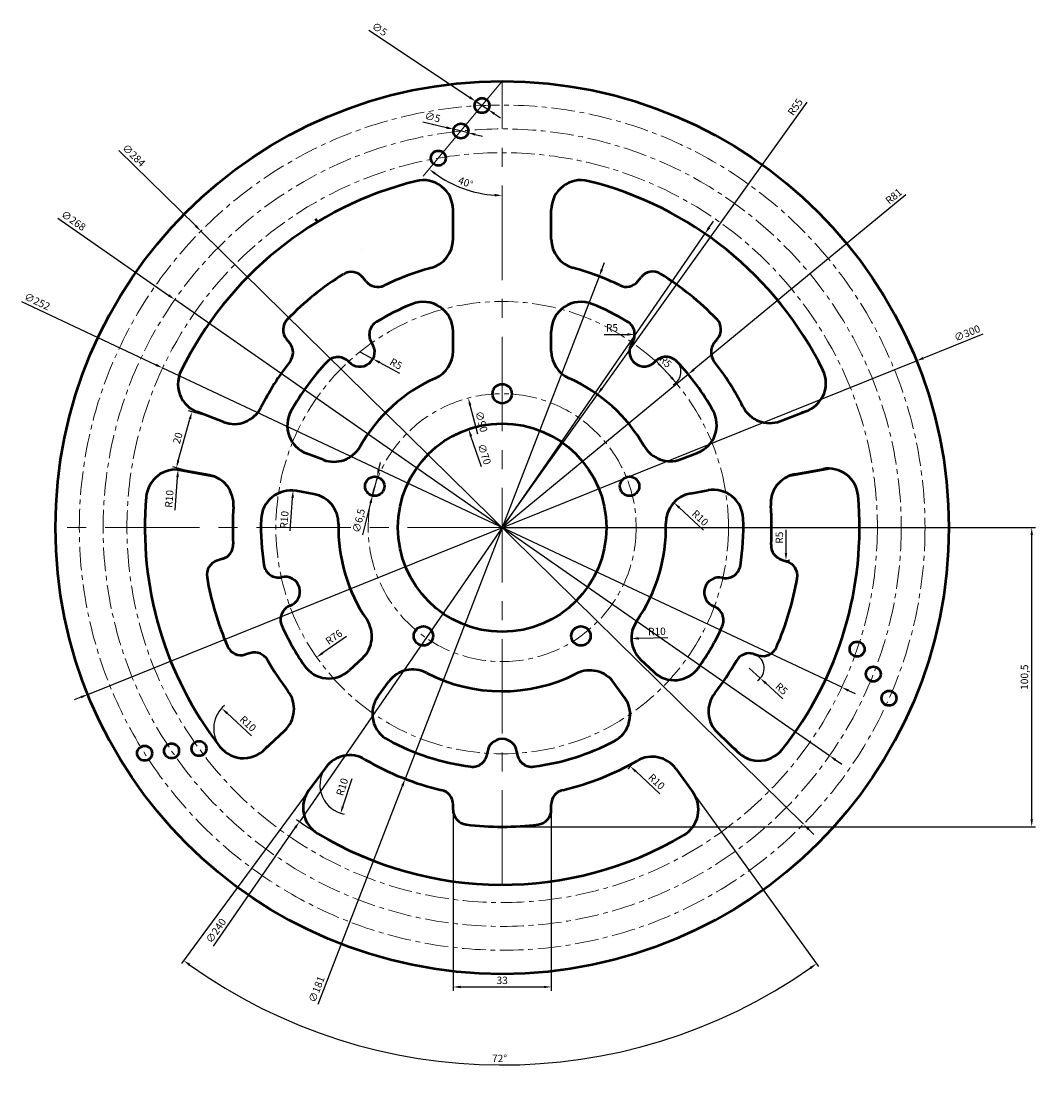
# Model space of a CAD drawing. Units: millimetres. Extents: x 2992 to 3333, y 1221 to 1583.
import ezdxf

# ---------------------------------------------------------------- set-up
doc = ezdxf.new("R2010")
doc.units = ezdxf.units.MM
doc.linetypes.add('CENTER', pattern=[50.8, 31.75, -6.35, 6.35, -6.35])
for name, color, linetype, lineweight in [('M-CNTR', 4, 'CENTER', 18), ('M-CONS', 8, 'Continuous', 13), ('M-DIMS', 2, 'Continuous', 25), ('M-OUTL', 7, 'Continuous', 50)]:
    doc.layers.add(name, color=color, linetype=linetype, lineweight=lineweight)
doc.styles.get("Standard").update_dxf_attribs({"font": 'arial.ttf'})
doc.dimstyles.new('ISO-25', dxfattribs={"dimtxt": 2.5, "dimasz": 2.5, "dimexe": 1.25, "dimexo": 0.625, "dimtad": 1, "dimtxsty": 'Standard', "dimcen": 2.5, "dimadec": 0, "dimazin": 0, "dimtfac": 1, "dimtmove": 0, "dimatfit": 3, "dimfxl": 1, "dimarcsym": 0})

# ---------------------------------------------------------------- blocks, each defined once
blk = doc.blocks.new('*D1')
at = {"layer": 'Defpoints', "color": 0, "transparency": 16777216}
for p in [(3137.05, 1317.59), (3170.04, 1317.59), (3170.04, 1258.36)]:
    blk.add_point(p, dxfattribs=at)
at = {"layer": 'M-DIMS', "color": 0, "lineweight": -2, "transparency": 16777216}
for p, q in [((3137.05, 1316.96), (3137.05, 1257.11)), ((3170.04, 1316.96), (3170.04, 1257.11)), ((3139.55, 1258.36), (3167.54, 1258.36))]:
    blk.add_line(p, q, dxfattribs=at)
at = {"layer": 'M-DIMS', "color": 0, "transparency": 16777216}
for points in [[(3139.55, 1258.77), (3139.55, 1257.94), (3137.05, 1258.36)], [(3167.54, 1258.77), (3167.54, 1257.94), (3170.04, 1258.36)]]:
    blk.add_solid(points, dxfattribs=at)
at = {"layer": 'M-DIMS', "color": 0, "transparency": 16777216, "insert": (3153.54, 1260.26), "char_height": 2.5, "attachment_point": 5}
blk.add_mtext('33', dxfattribs=at)
blk = doc.blocks.new('*D2')
at = {"layer": 'Defpoints', "color": 0, "transparency": 16777216}
for p in [(3049.35, 1451.62), (3055.58, 1449.88), (3050.33, 1431.07)]:
    blk.add_point(p, dxfattribs=at)
at = {"layer": 'M-DIMS', "color": 0, "lineweight": -2, "transparency": 16777216}
for p, q in [((3054.98, 1450.05), (3048.15, 1451.95)), ((3044.78, 1435.21), (3048.68, 1449.21)), ((3049.73, 1431.24), (3042.9, 1433.14))]:
    blk.add_line(p, q, dxfattribs=at)
at = {"layer": 'M-DIMS', "color": 0, "transparency": 16777216}
for points in [[(3048.28, 1449.32), (3049.08, 1449.1), (3049.35, 1451.62)], [(3044.38, 1435.33), (3045.18, 1435.1), (3044.1, 1432.81)]]:
    blk.add_solid(points, dxfattribs=at)
at = {"layer": 'M-DIMS', "color": 0, "transparency": 16777216, "insert": (3044.9, 1442.72), "char_height": 2.5, "attachment_point": 5, "rotation": 74.4122}
blk.add_mtext('20', dxfattribs=at)
blk = doc.blocks.new('*D3')
at = {"layer": 'Defpoints', "color": 0, "transparency": 16777216}
for p in [(3153.54, 1412.71), (3331.37, 1412.71), (3153.54, 1312.21)]:
    blk.add_point(p, dxfattribs=at)
at = {"layer": 'M-DIMS', "color": 0, "lineweight": -2, "transparency": 16777216}
for p, q in [((3154.16, 1412.71), (3332.62, 1412.71)), ((3331.37, 1314.71), (3331.37, 1410.21)), ((3154.16, 1312.21), (3332.62, 1312.21))]:
    blk.add_line(p, q, dxfattribs=at)
at = {"layer": 'M-DIMS', "color": 0, "transparency": 16777216}
for points in [[(3330.96, 1410.21), (3331.79, 1410.21), (3331.37, 1412.71)], [(3330.96, 1314.71), (3331.79, 1314.71), (3331.37, 1312.21)]]:
    blk.add_solid(points, dxfattribs=at)
at = {"layer": 'M-DIMS', "color": 0, "transparency": 16777216, "insert": (3329.25, 1362.46), "char_height": 2.5, "attachment_point": 5, "rotation": 90}
blk.add_mtext('100,5', dxfattribs=at)
blk = doc.blocks.new('*D4')
at = {"layer": 'Defpoints', "color": 0, "transparency": 16777216}
for p in [(3292.68, 1468.75), (3014.4, 1356.66)]:
    blk.add_point(p, dxfattribs=at)
at = {"layer": 'M-DIMS', "color": 0, "lineweight": -2, "transparency": 16777216}
for p, q in [((3314.94, 1477.72), (3294.99, 1469.69)), ((3014.4, 1356.66), (3292.68, 1468.75)), ((3012.08, 1355.73), (3009.76, 1354.8))]:
    blk.add_line(p, q, dxfattribs=at)
at = {"layer": 'M-DIMS', "color": 0, "transparency": 16777216}
for points in [[(3294.84, 1470.07), (3295.15, 1469.3), (3292.68, 1468.75)], [(3011.93, 1356.12), (3012.24, 1355.34), (3014.4, 1356.66)]]:
    blk.add_solid(points, dxfattribs=at)
at = {"layer": 'M-DIMS', "color": 0, "transparency": 16777216, "insert": (3309.8, 1477.78), "char_height": 2.5, "attachment_point": 5, "rotation": 21.9393}
blk.add_mtext('∅300', dxfattribs=at)
blk = doc.blocks.new('*D5')
at = {"layer": 'Defpoints', "color": 0, "transparency": 16777216}
for p in [(3144.69, 1555.93), (3148.85, 1553.16)]:
    blk.add_point(p, dxfattribs=at)
at = {"layer": 'M-DIMS', "color": 0, "lineweight": -2, "transparency": 16777216}
for p, q in [((3108.77, 1579.86), (3142.6, 1557.32)), ((3148.85, 1553.16), (3144.69, 1555.93)), ((3150.93, 1551.77), (3153.01, 1550.39))]:
    blk.add_line(p, q, dxfattribs=at)
at = {"layer": 'M-DIMS', "color": 0, "transparency": 16777216}
for points in [[(3142.84, 1557.67), (3142.37, 1556.97), (3144.69, 1555.93)], [(3151.16, 1552.12), (3150.7, 1551.43), (3148.85, 1553.16)]]:
    blk.add_solid(points, dxfattribs=at)
at = {"layer": 'M-DIMS', "color": 0, "transparency": 16777216, "insert": (3112.2, 1579.94), "char_height": 2.5, "attachment_point": 5, "rotation": 326.3304}
blk.add_mtext('∅5', dxfattribs=at)
blk = doc.blocks.new('*D6')
at = {"layer": 'Defpoints', "color": 0, "transparency": 16777216}
for p in [(3052.39, 1512.37), (3254.69, 1313.05)]:
    blk.add_point(p, dxfattribs=at)
at = {"layer": 'M-DIMS', "color": 0, "lineweight": -2, "transparency": 16777216}
for p, q in [((3024.86, 1539.49), (3050.61, 1514.13)), ((3254.69, 1313.05), (3052.39, 1512.37)), ((3256.47, 1311.29), (3258.25, 1309.54))]:
    blk.add_line(p, q, dxfattribs=at)
at = {"layer": 'M-DIMS', "color": 0, "transparency": 16777216}
for points in [[(3050.9, 1514.42), (3050.31, 1513.83), (3052.39, 1512.37)], [(3256.76, 1311.59), (3256.18, 1310.99), (3254.69, 1313.05)]]:
    blk.add_solid(points, dxfattribs=at)
at = {"layer": 'M-DIMS', "color": 0, "transparency": 16777216, "insert": (3029.62, 1537.57), "char_height": 2.5, "attachment_point": 5, "rotation": 315.4245}
blk.add_mtext('∅284', dxfattribs=at)
blk = doc.blocks.new('*D7')
at = {"layer": 'Defpoints', "color": 0, "transparency": 16777216}
for p in [(3043.61, 1489.34), (3263.46, 1336.07)]:
    blk.add_point(p, dxfattribs=at)
at = {"layer": 'M-DIMS', "color": 0, "lineweight": -2, "transparency": 16777216}
for p, q in [((3004.36, 1516.71), (3041.56, 1490.77)), ((3263.46, 1336.07), (3043.61, 1489.34)), ((3265.51, 1334.64), (3267.56, 1333.21))]:
    blk.add_line(p, q, dxfattribs=at)
at = {"layer": 'M-DIMS', "color": 0, "transparency": 16777216}
for points in [[(3041.8, 1491.11), (3041.33, 1490.43), (3043.61, 1489.34)], [(3265.75, 1334.99), (3265.27, 1334.3), (3263.46, 1336.07)]]:
    blk.add_solid(points, dxfattribs=at)
at = {"layer": 'M-DIMS', "color": 0, "transparency": 16777216, "insert": (3009.39, 1515.61), "char_height": 2.5, "attachment_point": 5, "rotation": 325.1175}
blk.add_mtext('∅268', dxfattribs=at)
blk = doc.blocks.new('*D8')
at = {"layer": 'Defpoints', "color": 0, "transparency": 16777216}
for p in [(3039.53, 1466.35), (3267.55, 1359.06)]:
    blk.add_point(p, dxfattribs=at)
at = {"layer": 'M-DIMS', "color": 0, "lineweight": -2, "transparency": 16777216}
for p, q in [((2992.14, 1488.66), (3037.27, 1467.42)), ((3267.55, 1359.06), (3039.53, 1466.35)), ((3269.81, 1358), (3272.07, 1356.93))]:
    blk.add_line(p, q, dxfattribs=at)
at = {"layer": 'M-DIMS', "color": 0, "transparency": 16777216}
for points in [[(3037.44, 1467.8), (3037.09, 1467.04), (3039.53, 1466.35)], [(3269.99, 1358.37), (3269.63, 1357.62), (3267.55, 1359.06)]]:
    blk.add_solid(points, dxfattribs=at)
at = {"layer": 'M-DIMS', "color": 0, "transparency": 16777216, "insert": (2997.26, 1488.42), "char_height": 2.5, "attachment_point": 5, "rotation": 334.8007}
blk.add_mtext('∅252', dxfattribs=at)
blk = doc.blocks.new('*D9')
at = {"layer": 'Defpoints', "color": 0, "transparency": 16777216}
for p in [(3221.63, 1511.52), (3085.45, 1313.9)]:
    blk.add_point(p, dxfattribs=at)
at = {"layer": 'M-DIMS', "color": 0, "lineweight": -2, "transparency": 16777216}
for p, q in [((3223.05, 1513.58), (3224.46, 1515.64)), ((3221.63, 1511.52), (3085.45, 1313.9)), ((3056.62, 1272.06), (3084.03, 1311.84))]:
    blk.add_line(p, q, dxfattribs=at)
blk.add_arc((3153.54, 1412.71), 120, 234.8334, 238.5826, dxfattribs=at)
at = {"layer": 'M-DIMS', "color": 0, "transparency": 16777216}
for points in [[(3222.7, 1513.82), (3223.39, 1513.34), (3221.63, 1511.52)], [(3083.69, 1312.07), (3084.37, 1311.6), (3085.45, 1313.9)]]:
    blk.add_solid(points, dxfattribs=at)
at = {"layer": 'M-DIMS', "color": 0, "transparency": 16777216, "insert": (3057.69, 1277.09), "char_height": 2.5, "attachment_point": 5, "rotation": 55.4302}
blk.add_mtext('∅240', dxfattribs=at)
blk = doc.blocks.new('*D10')
at = {"layer": 'Defpoints', "color": 0, "transparency": 16777216}
for p in [(3186.12, 1497.14), (3120.95, 1328.28)]:
    blk.add_point(p, dxfattribs=at)
at = {"layer": 'M-DIMS', "color": 0, "lineweight": -2, "transparency": 16777216}
for p, q in [((3187.02, 1499.47), (3187.92, 1501.8)), ((3186.12, 1497.14), (3120.95, 1328.28)), ((3091.73, 1252.54), (3120.05, 1325.95))]:
    blk.add_line(p, q, dxfattribs=at)
at = {"layer": 'M-DIMS', "color": 0, "transparency": 16777216}
for points in [[(3186.63, 1499.62), (3187.41, 1499.32), (3186.12, 1497.14)], [(3119.67, 1326.1), (3120.44, 1325.79), (3120.95, 1328.28)]]:
    blk.add_solid(points, dxfattribs=at)
at = {"layer": 'M-DIMS', "color": 0, "transparency": 16777216, "insert": (3091.51, 1257.46), "char_height": 2.5, "attachment_point": 5, "rotation": 68.8971}
blk.add_mtext('∅181', dxfattribs=at)
blk = doc.blocks.new('*D11')
at = {"layer": 'Defpoints', "color": 0, "transparency": 16777216}
for p in [(3105.74, 1471.79), (3110.14, 1469.42)]:
    blk.add_point(p, dxfattribs=at)
at = {"layer": 'M-DIMS', "color": 0, "lineweight": -2, "transparency": 16777216}
for p, q in [((3105.74, 1471.79), (3110.14, 1469.42)), ((3119.2, 1464.53), (3112.34, 1468.23))]:
    blk.add_line(p, q, dxfattribs=at)
at = {"layer": 'M-DIMS', "color": 0, "transparency": 16777216}
blk.add_solid([(3112.54, 1468.6), (3112.14, 1467.87), (3110.14, 1469.42)], dxfattribs=at)
at = {"layer": 'M-DIMS', "color": 0, "transparency": 16777216, "insert": (3117.77, 1467.46), "char_height": 2.5, "attachment_point": 5, "rotation": 331.6611}
blk.add_mtext('R5', dxfattribs=at)
blk = doc.blocks.new('*D12')
at = {"layer": 'Defpoints', "color": 0, "transparency": 16777216}
for p in [(3193.06, 1477.62), (3198.06, 1477.62)]:
    blk.add_point(p, dxfattribs=at)
at = {"layer": 'M-DIMS', "color": 0, "lineweight": -2, "transparency": 16777216}
blk.add_line((3187.76, 1477.62), (3195.56, 1477.62), dxfattribs=at)
at = {"layer": 'M-DIMS', "color": 0, "transparency": 16777216}
blk.add_solid([(3195.56, 1478.04), (3195.56, 1477.21), (3198.06, 1477.62)], dxfattribs=at)
at = {"layer": 'M-DIMS', "color": 0, "transparency": 16777216, "insert": (3190.41, 1479.52), "char_height": 2.5, "attachment_point": 5}
blk.add_mtext('R5', dxfattribs=at)
blk = doc.blocks.new('*D13')
at = {"layer": 'Defpoints', "color": 0, "transparency": 16777216}
for p in [(3208.59, 1465.1), (3211.98, 1461.42)]:
    blk.add_point(p, dxfattribs=at)
at = {"layer": 'M-DIMS', "color": 0, "lineweight": -2, "transparency": 16777216}
blk.add_line((3205.01, 1469), (3210.29, 1463.26), dxfattribs=at)
blk.add_arc((3208.59, 1465.1), 5, 298.2777, 36.4174, dxfattribs=at)
at = {"layer": 'M-DIMS', "color": 0, "transparency": 16777216}
blk.add_solid([(3210.59, 1463.54), (3209.98, 1462.98), (3211.98, 1461.42)], dxfattribs=at)
at = {"layer": 'M-DIMS', "color": 0, "transparency": 16777216, "insert": (3208.2, 1468.33), "char_height": 2.5, "attachment_point": 5, "rotation": 312.6017}
blk.add_mtext('R5', dxfattribs=at)
blk = doc.blocks.new('*D14')
at = {"layer": 'Defpoints', "color": 0, "transparency": 16777216}
for p in [(3211.19, 1421.13), (3218.52, 1414.33)]:
    blk.add_point(p, dxfattribs=at)
at = {"layer": 'M-DIMS', "color": 0, "lineweight": -2, "transparency": 16777216}
blk.add_line((3221.16, 1411.87), (3213.02, 1419.43), dxfattribs=at)
at = {"layer": 'M-DIMS', "color": 0, "transparency": 16777216}
blk.add_solid([(3213.3, 1419.73), (3212.74, 1419.12), (3211.19, 1421.13)], dxfattribs=at)
at = {"layer": 'M-DIMS', "color": 0, "transparency": 16777216, "insert": (3219.81, 1415.72), "char_height": 2.5, "attachment_point": 5, "rotation": 317.1429}
blk.add_mtext('R10', dxfattribs=at)
blk = doc.blocks.new('*D15')
at = {"layer": 'Defpoints', "color": 0, "transparency": 16777216}
for p in [(3196.93, 1375.45), (3206.93, 1375.64)]:
    blk.add_point(p, dxfattribs=at)
at = {"layer": 'M-DIMS', "color": 0, "lineweight": -2, "transparency": 16777216}
blk.add_line((3209.15, 1375.68), (3199.43, 1375.5), dxfattribs=at)
at = {"layer": 'M-DIMS', "color": 0, "transparency": 16777216}
blk.add_solid([(3199.42, 1375.92), (3199.44, 1375.08), (3196.93, 1375.45)], dxfattribs=at)
at = {"layer": 'M-DIMS', "color": 0, "transparency": 16777216, "insert": (3205.5, 1377.51), "char_height": 2.5, "attachment_point": 5, "rotation": 1.0474}
blk.add_mtext('R10', dxfattribs=at)
blk = doc.blocks.new('*D16')
at = {"layer": 'Defpoints', "color": 0, "transparency": 16777216}
for p in [(3153.54, 1412.71), (3091.25, 1369.16)]:
    blk.add_point(p, dxfattribs=at)
at = {"layer": 'M-DIMS', "color": 0, "lineweight": -2, "transparency": 16777216}
blk.add_line((3101.27, 1376.17), (3093.3, 1370.59), dxfattribs=at)
at = {"layer": 'M-DIMS', "color": 0, "transparency": 16777216}
blk.add_solid([(3093.06, 1370.94), (3093.54, 1370.25), (3091.25, 1369.16)], dxfattribs=at)
at = {"layer": 'M-DIMS', "color": 0, "transparency": 16777216, "insert": (3097.22, 1375.65), "char_height": 2.5, "attachment_point": 5, "rotation": 34.9576}
blk.add_mtext('R76', dxfattribs=at)
blk = doc.blocks.new('*D17')
at = {"layer": 'Defpoints', "color": 0, "transparency": 16777216}
for p in [(3083.33, 1425.15), (3082.58, 1415.17)]:
    blk.add_point(p, dxfattribs=at)
at = {"layer": 'M-DIMS', "color": 0, "lineweight": -2, "transparency": 16777216}
blk.add_line((3082.31, 1411.58), (3083.14, 1422.65), dxfattribs=at)
at = {"layer": 'M-DIMS', "color": 0, "transparency": 16777216}
blk.add_solid([(3082.73, 1422.69), (3083.56, 1422.62), (3083.33, 1425.15)], dxfattribs=at)
at = {"layer": 'M-DIMS', "color": 0, "transparency": 16777216, "insert": (3080.69, 1415.32), "char_height": 2.5, "attachment_point": 5, "rotation": 85.7143}
blk.add_mtext('R10', dxfattribs=at)
blk = doc.blocks.new('*D18')
at = {"layer": 'Defpoints', "color": 0, "transparency": 16777216}
for p in [(3044.7, 1432.18), (3043.95, 1422.2)]:
    blk.add_point(p, dxfattribs=at)
at = {"layer": 'M-DIMS', "color": 0, "lineweight": -2, "transparency": 16777216}
blk.add_line((3043.68, 1418.61), (3044.51, 1429.68), dxfattribs=at)
at = {"layer": 'M-DIMS', "color": 0, "transparency": 16777216}
blk.add_solid([(3044.09, 1429.72), (3044.93, 1429.65), (3044.7, 1432.18)], dxfattribs=at)
at = {"layer": 'M-DIMS', "color": 0, "transparency": 16777216, "insert": (3042.05, 1422.35), "char_height": 2.5, "attachment_point": 5, "rotation": 85.7143}
blk.add_mtext('R10', dxfattribs=at)
blk = doc.blocks.new('*D19')
at = {"layer": 'Defpoints', "color": 0, "transparency": 16777216}
for p in [(3059.34, 1352.03), (3066.67, 1345.23)]:
    blk.add_point(p, dxfattribs=at)
at = {"layer": 'M-DIMS', "color": 0, "lineweight": -2, "transparency": 16777216}
blk.add_line((3069.31, 1342.78), (3061.17, 1350.33), dxfattribs=at)
blk.add_arc((3066.67, 1345.23), 10, 129.9809, 214.2575, dxfattribs=at)
at = {"layer": 'M-DIMS', "color": 0, "transparency": 16777216}
blk.add_solid([(3061.45, 1350.64), (3060.89, 1350.03), (3059.34, 1352.03)], dxfattribs=at)
at = {"layer": 'M-DIMS', "color": 0, "transparency": 16777216, "insert": (3067.96, 1346.62), "char_height": 2.5, "attachment_point": 5, "rotation": 317.1429}
blk.add_mtext('R10', dxfattribs=at)
blk = doc.blocks.new('*D20')
at = {"layer": 'Defpoints', "color": 0, "transparency": 16777216}
for p in [(3102.34, 1326.23), (3099.28, 1316.71)]:
    blk.add_point(p, dxfattribs=at)
at = {"layer": 'M-DIMS', "color": 0, "lineweight": -2, "transparency": 16777216}
blk.add_line((3103.02, 1328.33), (3100.04, 1319.09), dxfattribs=at)
blk.add_arc((3102.34, 1326.23), 10, 147.246, 259.3056, dxfattribs=at)
at = {"layer": 'M-DIMS', "color": 0, "transparency": 16777216}
blk.add_solid([(3099.65, 1319.21), (3100.44, 1318.96), (3099.28, 1316.71)], dxfattribs=at)
at = {"layer": 'M-DIMS', "color": 0, "transparency": 16777216, "insert": (3100.11, 1325.48), "char_height": 2.5, "attachment_point": 5, "rotation": 72.1436}
blk.add_mtext('R10', dxfattribs=at)
blk = doc.blocks.new('*D21')
at = {"layer": 'Defpoints', "color": 0, "transparency": 16777216}
for p in [(3196.54, 1332.52), (3203.87, 1325.72)]:
    blk.add_point(p, dxfattribs=at)
at = {"layer": 'M-DIMS', "color": 0, "lineweight": -2, "transparency": 16777216}
blk.add_line((3206.52, 1323.27), (3198.37, 1330.82), dxfattribs=at)
blk.add_arc((3203.87, 1325.72), 10, 123.6362, 144.3048, dxfattribs=at)
at = {"layer": 'M-DIMS', "color": 0, "transparency": 16777216}
blk.add_solid([(3198.66, 1331.13), (3198.09, 1330.52), (3196.54, 1332.52)], dxfattribs=at)
at = {"layer": 'M-DIMS', "color": 0, "transparency": 16777216, "insert": (3205.17, 1327.11), "char_height": 2.5, "attachment_point": 5, "rotation": 317.1429}
blk.add_mtext('R10', dxfattribs=at)
blk = doc.blocks.new('*D22')
at = {"layer": 'Defpoints', "color": 0, "transparency": 16777216}
for p in [(3248.85, 1406.68), (3248.85, 1401.68)]:
    blk.add_point(p, dxfattribs=at)
at = {"layer": 'M-DIMS', "color": 0, "lineweight": -2, "transparency": 16777216}
blk.add_line((3248.85, 1411.98), (3248.85, 1404.18), dxfattribs=at)
blk.add_arc((3248.85, 1406.68), 5, 260.5307, 284.3239, dxfattribs=at)
at = {"layer": 'M-DIMS', "color": 0, "transparency": 16777216}
blk.add_solid([(3248.43, 1404.18), (3249.26, 1404.18), (3248.85, 1401.68)], dxfattribs=at)
at = {"layer": 'M-DIMS', "color": 0, "transparency": 16777216, "insert": (3246.95, 1409.33), "char_height": 2.5, "attachment_point": 5, "rotation": 90}
blk.add_mtext('R5', dxfattribs=at)
blk = doc.blocks.new('*D23')
at = {"layer": 'Defpoints', "color": 0, "transparency": 16777216}
for p in [(3236.54, 1365.48), (3240.23, 1362.1)]:
    blk.add_point(p, dxfattribs=at)
at = {"layer": 'M-DIMS', "color": 0, "lineweight": -2, "transparency": 16777216}
for p, q in [((3236.54, 1365.48), (3240.23, 1362.1)), ((3247.83, 1355.15), (3242.08, 1360.42))]:
    blk.add_line(p, q, dxfattribs=at)
blk.add_arc((3236.54, 1365.48), 5, 303.2437, 66.2068, dxfattribs=at)
at = {"layer": 'M-DIMS', "color": 0, "transparency": 16777216}
blk.add_solid([(3242.36, 1360.72), (3241.8, 1360.11), (3240.23, 1362.1)], dxfattribs=at)
at = {"layer": 'M-DIMS', "color": 0, "transparency": 16777216, "insert": (3247.16, 1358.34), "char_height": 2.5, "attachment_point": 5, "rotation": 317.5677}
blk.add_mtext('R5', dxfattribs=at)
blk = doc.blocks.new('*D24')
at = {"layer": 'Defpoints', "color": 0, "transparency": 16777216}
for p in [(3216.02, 1464.25), (3153.54, 1412.71)]:
    blk.add_point(p, dxfattribs=at)
at = {"layer": 'M-DIMS', "color": 0, "lineweight": -2, "transparency": 16777216}
for p, q in [((3289.05, 1524.5), (3217.95, 1465.84)), ((3153.54, 1412.71), (3216.02, 1464.25))]:
    blk.add_line(p, q, dxfattribs=at)
at = {"layer": 'M-DIMS', "color": 0, "transparency": 16777216}
blk.add_solid([(3217.68, 1466.17), (3218.21, 1465.52), (3216.02, 1464.25)], dxfattribs=at)
at = {"layer": 'M-DIMS', "color": 0, "transparency": 16777216, "insert": (3285.24, 1523.82), "char_height": 2.5, "attachment_point": 5, "rotation": 39.5211}
blk.add_mtext('R81', dxfattribs=at)
blk = doc.blocks.new('*D25')
at = {"layer": 'Defpoints', "color": 0, "transparency": 16777216}
for p in [(3185.55, 1457.44), (3153.54, 1412.71)]:
    blk.add_point(p, dxfattribs=at)
at = {"layer": 'M-DIMS', "color": 0, "lineweight": -2, "transparency": 16777216}
for p, q in [((3255.88, 1555.72), (3187, 1459.47)), ((3153.54, 1412.71), (3185.55, 1457.44))]:
    blk.add_line(p, q, dxfattribs=at)
at = {"layer": 'M-DIMS', "color": 0, "transparency": 16777216}
blk.add_solid([(3186.66, 1459.71), (3187.34, 1459.23), (3185.55, 1457.44)], dxfattribs=at)
at = {"layer": 'M-DIMS', "color": 0, "transparency": 16777216, "insert": (3252.23, 1553.88), "char_height": 2.5, "attachment_point": 5, "rotation": 54.4123}
blk.add_mtext('R55', dxfattribs=at)
blk = doc.blocks.new('*D26')
at = {"layer": 'Defpoints', "color": 0, "transparency": 16777216}
for p in [(3142.26, 1445.84), (3164.81, 1379.57)]:
    blk.add_point(p, dxfattribs=at)
at = {"layer": 'M-DIMS', "color": 0, "lineweight": -2, "transparency": 16777216}
blk.add_line((3146.6, 1433.09), (3143.07, 1443.47), dxfattribs=at)
at = {"layer": 'M-DIMS', "color": 0, "transparency": 16777216}
blk.add_solid([(3143.46, 1443.61), (3142.67, 1443.34), (3142.26, 1445.84)], dxfattribs=at)
at = {"layer": 'M-DIMS', "color": 0, "transparency": 16777216, "insert": (3147.25, 1437.3), "char_height": 2.5, "attachment_point": 5, "rotation": 288.7953}
blk.add_mtext('∅70', dxfattribs=at)
blk = doc.blocks.new('*D27')
at = {"layer": 'Defpoints', "color": 0, "transparency": 16777216}
for p in [(3142.15, 1456.24), (3164.92, 1369.17)]:
    blk.add_point(p, dxfattribs=at)
at = {"layer": 'M-DIMS', "color": 0, "lineweight": -2, "transparency": 16777216}
blk.add_line((3145.33, 1444.11), (3142.79, 1453.83), dxfattribs=at)
at = {"layer": 'M-DIMS', "color": 0, "transparency": 16777216}
blk.add_solid([(3143.19, 1453.93), (3142.38, 1453.72), (3142.15, 1456.24)], dxfattribs=at)
at = {"layer": 'M-DIMS', "color": 0, "transparency": 16777216, "insert": (3146.28, 1448.26), "char_height": 2.5, "attachment_point": 5, "rotation": 284.6536}
blk.add_mtext('∅90', dxfattribs=at)
blk = doc.blocks.new('*D28')
at = {"layer": 'Defpoints', "color": 0, "transparency": 16777216}
for p in [(3094.29, 1332.15), (3211.99, 1331.57), (3088.63, 1324.46), (3217.56, 1323.82), (3115.07, 1236.28)]:
    blk.add_point(p, dxfattribs=at)
at = {"layer": 'M-DIMS', "color": 0, "lineweight": -2, "transparency": 16777216}
for p, q in [((3088.26, 1323.96), (3045.81, 1266.24)), ((3217.93, 1323.31), (3259.81, 1265.18))]:
    blk.add_line(p, q, dxfattribs=at)
blk.add_arc((3153.54, 1412.71), 180.57, 234.4583, 304.9725, dxfattribs=at)
at = {"layer": 'M-DIMS', "color": 0, "transparency": 16777216}
for points in [[(3048.33, 1265.44), (3048.82, 1266.12), (3046.55, 1267.25)], [(3256.8, 1265.08), (3257.28, 1264.4), (3259.08, 1266.19)]]:
    blk.add_solid(points, dxfattribs=at)
at = {"layer": 'M-DIMS', "color": 0, "transparency": 16777216, "insert": (3152.65, 1234.02), "char_height": 2.5, "attachment_point": 5, "rotation": 359.7154}
blk.add_mtext('72°', dxfattribs=at)
blk = doc.blocks.new('*D29')
at = {"layer": 'Defpoints', "color": 0, "transparency": 16777216}
for p in [(3111.51, 1429.77), (3109.97, 1423.46)]:
    blk.add_point(p, dxfattribs=at)
at = {"layer": 'M-DIMS', "color": 0, "lineweight": -2, "transparency": 16777216}
for p, q in [((3112.1, 1432.2), (3112.69, 1434.63)), ((3111.51, 1429.77), (3109.97, 1423.46)), ((3106.77, 1410.3), (3109.38, 1421.03))]:
    blk.add_line(p, q, dxfattribs=at)
at = {"layer": 'M-DIMS', "color": 0, "transparency": 16777216}
for points in [[(3111.7, 1432.3), (3112.51, 1432.1), (3111.51, 1429.77)], [(3108.97, 1421.13), (3109.78, 1420.93), (3109.97, 1423.46)]]:
    blk.add_solid(points, dxfattribs=at)
at = {"layer": 'M-DIMS', "color": 0, "transparency": 16777216, "insert": (3105.67, 1414.96), "char_height": 2.5, "attachment_point": 5, "rotation": 76.3045}
blk.add_mtext('∅6,5', dxfattribs=at)
blk = doc.blocks.new('*D30')
at = {"layer": 'Defpoints', "color": 0, "transparency": 16777216}
for p in [(3153.54, 1562.71), (3153.54, 1562.71), (3127.04, 1530.77), (3136.45, 1528.36), (3153.54, 1292.71)]:
    blk.add_point(p, dxfattribs=at)
at = {"layer": 'M-DIMS', "color": 0, "lineweight": -2, "transparency": 16777216}
blk.add_arc((3153.54, 1562.71), 38.36, 234.0489, 266.2656, dxfattribs=at)
at = {"layer": 'M-DIMS', "color": 0, "transparency": 16777216}
for points in [[(3130.76, 1531.32), (3131.27, 1531.98), (3129.04, 1533.18)], [(3151.05, 1524.84), (3151.03, 1524.01), (3153.54, 1524.34)]]:
    blk.add_solid(points, dxfattribs=at)
at = {"layer": 'M-DIMS', "color": 0, "transparency": 16777216, "insert": (3141.16, 1528.41), "char_height": 2.5, "attachment_point": 5, "rotation": 340.1573}
blk.add_mtext('40°', dxfattribs=at)
blk = doc.blocks.new('*D31')
at = {"layer": 'Defpoints', "color": 0, "transparency": 16777216}
for p in [(3137.23, 1546.57), (3142.09, 1545.4)]:
    blk.add_point(p, dxfattribs=at)
at = {"layer": 'M-DIMS', "color": 0, "lineweight": -2, "transparency": 16777216}
for p, q in [((3126.9, 1549.06), (3134.8, 1547.16)), ((3142.09, 1545.4), (3137.23, 1546.57)), ((3144.52, 1544.82), (3146.96, 1544.23))]:
    blk.add_line(p, q, dxfattribs=at)
at = {"layer": 'M-DIMS', "color": 0, "transparency": 16777216}
for points in [[(3134.9, 1547.56), (3134.71, 1546.75), (3137.23, 1546.57)], [(3144.62, 1545.22), (3144.43, 1544.41), (3142.09, 1545.4)]]:
    blk.add_solid(points, dxfattribs=at)
at = {"layer": 'M-DIMS', "color": 0, "transparency": 16777216, "insert": (3130.1, 1550.32), "char_height": 2.5, "attachment_point": 5, "rotation": 346.4454}
blk.add_mtext('∅5', dxfattribs=at)

msp = doc.modelspace()

# ---------------------------------------------------------------- linework, layer by layer
at = {"layer": 'M-CNTR'}
for p, q in [((3153.538, 1292.708), (3153.538, 1562.708)), ((3153.538, 1412.708), (3003.538, 1412.708)), ((3153.538, 1412.708), (3303.538, 1412.708))]:
    msp.add_line(p, q, dxfattribs=at)
at = {"layer": 'M-CNTR', "ltscale": 0.25, "transparency": 33554534}
for radius in [142, 134, 126, 76, 45]:
    msp.add_circle((3153.538, 1412.708), radius, dxfattribs=at)
at = {"layer": 'M-CONS'}
msp.add_line((3153.538, 1562.708), (3127.038, 1530.772), dxfattribs=at)
at = {"layer": 'M-OUTL'}
for p, q in [((3091.61, 1515.493), (3090.893, 1516.379)), ((3137.038, 1509.651), (3137.038, 1519.468)), ((3170.038, 1509.651), (3170.038, 1519.468)), ((3106.209, 1505.67), (3106.209, 1505.67)), ((3107.844, 1495.426), (3106.739, 1496.792)), ((3199.094, 1495.503), (3200.197, 1496.87)), ((3137.038, 1472.061), (3137.038, 1478.577)), ((3170.038, 1472.061), (3170.038, 1478.577)), ((3082.188, 1474.671), (3081.083, 1476.036)), ((3224.785, 1474.79), (3225.887, 1476.158)), ((3060.042, 1448.186), (3051.119, 1451.571)), ((3246.915, 1448.499), (3255.826, 1451.915)), ((3093.49, 1435.494), (3087.818, 1437.646)), ((3213.51, 1435.695), (3219.174, 1437.866)), ((3056.718, 1429.933), (3043.949, 1432.205)), ((3055.108, 1430.363), (3045.715, 1432.048)), ((3250.272, 1430.248), (3263.095, 1432.573)), ((3251.909, 1430.693), (3261.297, 1432.41)), ((3090.305, 1423.958), (3084.333, 1425.02)), ((3216.734, 1424.167), (3222.703, 1425.249)), ((3059.625, 1402.195), (3057.94, 1401.698)), ((3247.417, 1401.886), (3249.1, 1401.384)), ((3068.966, 1370.545), (3067.281, 1370.047)), ((3106.608, 1368.861), (3102.175, 1364.72)), ((3200.031, 1368.397), (3204.422, 1364.212)), ((3237.972, 1370.267), (3239.655, 1369.764)), ((3111.89, 1356.083), (3115.484, 1360.97)), ((3194.622, 1355.672), (3191.077, 1360.594)), ((3080.467, 1344.438), (3073.494, 1337.923)), ((3225.928, 1343.715), (3232.836, 1337.131)), ((3094.287, 1332.15), (3088.633, 1324.463)), ((3211.986, 1331.566), (3217.564, 1323.822)), ((3137.038, 1317.903), (3137.038, 1319.66)), ((3170.038, 1317.903), (3170.038, 1319.66))]:
    msp.add_line(p, q, dxfattribs=at)
for centre, radius in [((3153.538, 1412.708), 150), ((3146.766, 1554.546), 2.5), ((3139.664, 1545.988), 2.5), ((3132.099, 1536.871), 2.5), ((3153.538, 1457.708), 3.25), ((3153.538, 1412.708), 35), ((3110.741, 1426.614), 3.25), ((3196.336, 1426.614), 3.25), ((3127.088, 1376.302), 3.25), ((3179.989, 1376.302), 3.25), ((3272.738, 1371.873), 2.5), ((3278.178, 1363.505), 2.5), ((3283.455, 1355.388), 2.5), ((3033.464, 1336.904), 2.5), ((3042.507, 1337.687), 2.5), ((3051.72, 1338.485), 2.5)]:
    msp.add_circle(centre, radius, dxfattribs=at)
for centre, radius, start, end in [((3153.538, 1412.708), 120, 103.9402, 154.00461), ((3127.038, 1519.468), 10, 0, 103.9402), ((3180.038, 1519.468), 10, 76.0598, 180), ((3153.538, 1412.708), 120, 26.18769, 76.0598), ((3127.038, 1509.651), 10, 285.28863, 0), ((3180.038, 1509.651), 10, 180, 254.71137), ((3102.852, 1493.647), 5, 38.97241, 122.05613), ((3153.538, 1412.708), 90.5, 105.28863, 115.96183), ((3153.538, 1412.708), 90.5, 64.13432, 74.71137), ((3204.089, 1493.732), 5, 58.04002, 141.12374), ((3153.538, 1412.708), 100.5, 122.05613, 135.88868), ((3111.731, 1498.571), 5, 218.97241, 295.96183), ((3195.202, 1498.641), 5, 244.13432, 321.12374), ((3153.538, 1412.708), 100.5, 44.20747, 58.04002), ((3153.538, 1412.708), 81, 111.91554, 121.42804), ((3127.038, 1478.577), 10, 0, 111.91554), ((3180.038, 1478.577), 10, 68.08446, 180), ((3153.538, 1412.708), 81, 58.66811, 68.08446), ((3084.97, 1479.181), 5, 135.88868, 218.97241), ((3113.91, 1477.558), 5, 121.42804, 215.20022), ((3193.058, 1477.625), 5, 324.89593, 58.66811), ((3221.995, 1479.296), 5, 321.12374, 44.20747), ((3078.301, 1471.526), 5, 321.98298, 38.97241), ((3105.739, 1471.794), 5, 220.85748, 37.08734), ((3201.239, 1471.874), 5, 143.00881, 319.23867), ((3228.677, 1471.652), 5, 141.12374, 218.11317), ((3098.395, 1465.007), 5, 42.74459, 136.51678), ((3127.038, 1472.061), 10, 294.05995, 0), ((3180.038, 1472.061), 10, 180, 245.94005), ((3208.594, 1465.099), 5, 43.57938, 137.35156), ((3153.538, 1412.708), 90.5, 141.98298, 153.51), ((3153.538, 1412.708), 81, 136.51678, 151.12377), ((3153.538, 1412.708), 81, 29.06853, 43.57938), ((3153.538, 1412.708), 90.5, 26.6823, 38.11317), ((3252.247, 1461.252), 10, 280.36107, 26.18769), ((3054.667, 1460.921), 10, 154.00461, 259.83123), ((3153.538, 1412.708), 55, 114.05995, 150.37064), ((3153.538, 1412.708), 55, 29.82166, 65.94005), ((3063.59, 1457.535), 10, 249.22052, 333.51), ((3091.366, 1446.995), 10, 151.12377, 249.22052), ((3215.595, 1447.204), 10, 290.97178, 29.06853), ((3243.336, 1457.837), 10, 206.6823, 290.97178), ((3097.038, 1444.843), 10, 249.22052, 330.37064), ((3209.931, 1445.033), 10, 209.82166, 290.97178), ((3043.949, 1422.205), 10, 79.83123, 175.04714), ((3053.342, 1420.52), 10, 355.54176, 79.83123), ((3253.708, 1420.856), 10, 100.36107, 184.65054), ((3263.095, 1422.573), 10, 5.14516, 100.36107), ((3153.538, 1412.708), 120, 175.04714, 217.83844), ((3082.581, 1415.175), 10, 79.91209, 178.00884), ((3088.554, 1414.112), 10, 358.76197, 79.91209), ((3218.518, 1414.327), 10, 100.27716, 181.42727), ((3224.487, 1415.409), 10, 2.18041, 100.27716), ((3153.538, 1412.708), 120, 321.59238, 5.14516), ((3153.538, 1412.708), 90.5, 175.54176, 183.43221), ((3153.538, 1412.708), 90.5, 356.37935, 4.65054), ((3153.538, 1412.708), 81, 178.00884, 188.89842), ((3153.538, 1412.708), 81, 350.91314, 2.18041), ((3153.538, 1412.708), 55, 178.76197, 214.20446), ((3153.538, 1412.708), 55, 325.22636, 1.42727), ((3058.21, 1406.991), 5, 286.44279, 3.43221), ((3248.848, 1406.677), 5, 176.37935, 253.36877), ((3059.355, 1396.902), 5, 106.44279, 189.52651), ((3247.669, 1396.593), 5, 350.28505, 73.36877), ((3078.453, 1400.952), 5, 188.89842, 282.67061), ((3228.585, 1400.705), 5, 257.14095, 350.91314), ((3153.538, 1412.708), 100.5, 189.52651, 203.35907), ((3080.647, 1391.196), 5, 288.32786, 104.55772), ((3226.359, 1390.956), 5, 75.25384, 251.4837), ((3153.538, 1412.708), 100.5, 336.4525, 350.28505), ((3084.102, 1381.812), 5, 110.21497, 203.98716), ((3222.873, 1381.583), 5, 335.8244, 69.59659), ((3153.538, 1412.708), 81, 203.98716, 214.9576), ((3099.781, 1376.168), 10, 313.05435, 34.20446), ((3206.93, 1375.636), 10, 145.22636, 226.37648), ((3153.538, 1412.708), 81, 324.47323, 335.8244), ((3065.866, 1374.843), 5, 203.35907, 286.44279), ((3241.086, 1374.555), 5, 253.36877, 336.4525), ((3070.381, 1365.749), 5, 29.45337, 106.44279), ((3153.538, 1412.708), 90.5, 209.45337, 217.34382), ((3153.538, 1412.708), 90.5, 322.087, 330.3582), ((3236.541, 1365.476), 5, 73.36877, 150.3582), ((3095.348, 1372.027), 10, 214.9576, 313.05435), ((3123.54, 1355.044), 10, 62.51494, 143.66506), ((3182.963, 1354.749), 10, 35.76576, 116.91588), ((3211.321, 1371.451), 10, 226.37648, 324.47323), ((3153.538, 1412.708), 55, 242.51494, 296.91588), ((3073.64, 1351.745), 10, 313.05435, 37.34382), ((3232.827, 1350.954), 10, 142.087, 226.37648), ((3119.946, 1350.158), 10, 143.66506, 241.76181), ((3186.508, 1349.827), 10, 297.66901, 35.76576), ((3066.667, 1345.23), 10, 217.83844, 323.66506), ((3153.538, 1412.708), 81, 241.76181, 262.45563), ((3153.538, 1336.708), 5, 1.88507, 178.11493), ((3153.538, 1412.708), 81, 277.54437, 297.66901), ((3102.343, 1326.225), 10, 59.37558, 143.66506), ((3143.56, 1337.366), 5, 262.45563, 356.22782), ((3163.517, 1337.366), 5, 183.77218, 277.54437), ((3203.872, 1325.721), 10, 35.76576, 120.05524), ((3239.736, 1344.37), 10, 215.76576, 321.59238), ((3153.538, 1412.708), 90.5, 239.37558, 256.98942), ((3153.538, 1412.708), 90.5, 283.01058, 300.05524), ((3132.038, 1319.66), 5, 0, 76.98942), ((3175.038, 1319.66), 5, 103.01058, 180), ((3096.688, 1318.537), 10, 143.66506, 238.88097), ((3209.45, 1317.977), 10, 300.54986, 35.76576), ((3142.038, 1317.903), 5, 180, 263.08372), ((3165.038, 1317.903), 5, 276.91628, 0), ((3153.538, 1412.708), 100.5, 263.08372, 276.91628), ((3153.538, 1412.708), 120, 238.88097, 300.54986)]:
    msp.add_arc(centre, radius, start, end, dxfattribs=at)

# ---------------------------------------------------------------- dimensions: what is measured, and where the dimension line sits
at = {"layer": 'M-DIMS'}
for p1, p2, picture, middle in [((3148.847, 1553.16), (3144.685, 1555.932), '*D5', (3111.107, 1578.301)), ((3254.689, 1313.046), (3052.388, 1512.37), '*D6', (3028.237, 1536.166)), ((3263.462, 1336.074), (3043.615, 1489.342), '*D7', (3008.26, 1513.99)), ((3221.628, 1511.52), (3085.449, 1313.896), '*D9', (3059.313, 1275.967)), ((3186.122, 1497.139), (3120.954, 1328.277), '*D10', (3093.349, 1256.748)), ((3267.547, 1359.061), (3039.53, 1466.355), '*D8', (2996.421, 1486.64)), ((3014.401, 1356.664), (3292.675, 1468.752), '*D4', (3310.54, 1475.947)), ((3164.922, 1369.172), (3142.155, 1456.244), '*D27', (3144.373, 1447.758)), ((3164.815, 1379.574), (3142.262, 1445.842), '*D26', (3145.385, 1436.664))]:
    dim = msp.add_diameter_dim_2p(p1=p1, p2=p2, dimstyle='ISO-25', override={"dimclrd": 0, "dimclre": 0, "dimclrt": 0}, dxfattribs=at)
    dim.commit()
    dim.dimension.update_dxf_attribs({"geometry": picture, "text_midpoint": middle, "dimtype": 163})
for base, line1, line2, picture, middle in [((3136.446, 1528.362), ((3153.538, 1292.708), (3153.538, 1562.708)), ((3153.538, 1562.708), (3127.038, 1530.772)), '*D30', (3141.162, 1528.41)), ((3115.067, 1236.282), ((3211.986, 1331.566), (3217.564, 1323.822)), ((3094.287, 1332.15), (3088.633, 1324.463)), '*D28', (3152.651, 1234.018))]:
    dim = msp.add_angular_dim_2l(base=base, line1=line1, line2=line2, dimstyle='ISO-25', override={"dimclrd": 0, "dimclre": 0, "dimclrt": 0}, dxfattribs=at)
    dim.commit()
    dim.dimension.update_dxf_attribs({"geometry": picture, "text_midpoint": middle})
for center, mpoint, picture, middle in [((3153.538, 1412.708), (3185.546, 1457.435), '*D25', (3253.773, 1552.778)), ((3153.538, 1412.708), (3216.021, 1464.253), '*D24', (3286.452, 1522.356)), ((3193.058, 1477.625), (3198.058, 1477.625), '*D12', (3190.408, 1477.625)), ((3208.594, 1465.099), (3211.979, 1461.419), '*D13', (3206.801, 1467.05)), ((3043.949, 1422.205), (3044.696, 1432.177), '*D18', (3043.949, 1422.205)), ((3082.581, 1415.175), (3083.329, 1425.147), '*D17', (3082.581, 1415.175)), ((3218.518, 1414.327), (3211.188, 1421.129), '*D14', (3218.518, 1414.327)), ((3153.538, 1412.708), (3091.251, 1369.162), '*D16', (3098.308, 1374.096)), ((3248.848, 1406.677), (3248.848, 1401.677), '*D22', (3248.848, 1409.327)), ((3206.93, 1375.636), (3196.932, 1375.453), '*D15', (3205.538, 1375.611)), ((3066.667, 1345.23), (3059.336, 1352.032), '*D19', (3066.667, 1345.23)), ((3203.872, 1325.721), (3196.542, 1332.523), '*D21', (3203.872, 1325.721)), ((3102.343, 1326.225), (3099.277, 1316.707), '*D20', (3101.916, 1324.9))]:
    dim = msp.add_radius_dim(center=center, mpoint=mpoint, dimstyle='ISO-25', override={"dimclrd": 0, "dimclre": 0, "dimclrt": 0}, dxfattribs=at)
    dim.commit()
    dim.dimension.update_dxf_attribs({"geometry": picture, "text_midpoint": middle, "dimtype": 164})
for p1, p2, picture, middle in [((3142.095, 1545.402), (3137.234, 1546.574), '*D31', (3130.1, 1550.322)), ((3111.51, 1429.771), (3109.971, 1423.456), '*D29', (3105.67, 1414.963))]:
    dim = msp.add_diameter_dim_2p(p1=p1, p2=p2, dimstyle='ISO-25', override={"dimclrd": 0, "dimclre": 0, "dimclrt": 0}, dxfattribs=at)
    dim.commit()
    dim.dimension.update_dxf_attribs({"geometry": picture, "text_midpoint": middle})
for center, mpoint, picture, middle in [((3105.739, 1471.794), (3110.139, 1469.421), '*D11', (3117.773, 1467.458)), ((3236.541, 1365.476), (3240.231, 1362.102), '*D23', (3247.157, 1358.34))]:
    dim = msp.add_radius_dim(center=center, mpoint=mpoint, dimstyle='ISO-25', override={"dimclrd": 0, "dimclre": 0, "dimclrt": 0}, dxfattribs=at)
    dim.commit()
    dim.dimension.update_dxf_attribs({"geometry": picture, "text_midpoint": middle})
dim = msp.add_aligned_dim(p1=(3050.333, 1431.069), p2=(3055.581, 1449.878), distance=6.466, dimstyle='ISO-25', override={"dimdec": 0, "dimclrd": 0, "dimclre": 0, "dimclrt": 0}, dxfattribs=at)
dim.commit()
dim.dimension.update_dxf_attribs({"geometry": '*D2', "text_midpoint": (3044.897, 1442.722)})
dim = msp.add_linear_dim(base=(3331.373, 1412.708), p1=(3153.538, 1312.208), p2=(3153.538, 1412.708), angle=90, dimstyle='ISO-25', override={"dimclrd": 0, "dimclre": 0, "dimclrt": 0}, dxfattribs=at)
dim.commit()
dim.dimension.update_dxf_attribs({"geometry": '*D3', "text_midpoint": (3329.245, 1362.458)})
dim = msp.add_linear_dim(base=(3170.038, 1258.357), p1=(3137.048, 1317.59), p2=(3170.038, 1317.59), dimstyle='ISO-25', override={"dimdec": 0, "dimclrd": 0, "dimclre": 0, "dimclrt": 0}, dxfattribs=at)
dim.commit()
dim.dimension.update_dxf_attribs({"geometry": '*D1', "text_midpoint": (3153.543, 1260.259)})

doc.saveas('drawing.dxf')
